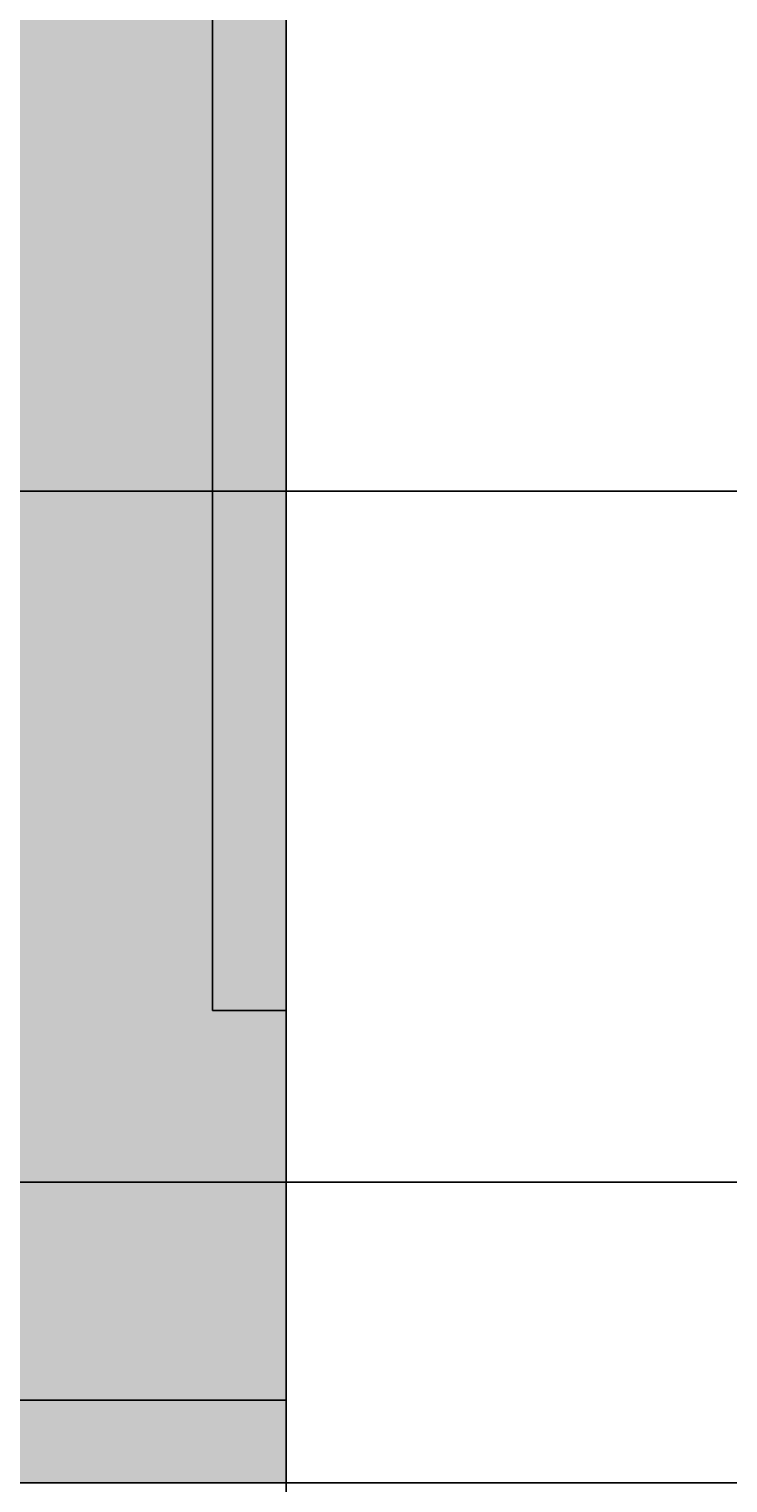
# Model space of a CAD drawing. Units: feet. Extents: x 2193 to 3502, y 890 to 1601.
# Tile 7 of 17: x 2710 to 2848, y 1073 to 1360. Entities that reach past the tile are written whole.
import ezdxf

# ---------------------------------------------------------------- set-up
doc = ezdxf.new("R2010")
doc.units = ezdxf.units.FT
for name, color, linetype, lineweight in [('A-ANNO-DIMS', 2, 'Continuous', 18), ('A-ELEV', 7, 'Continuous', 25), ('A-ELEV-PATT', 8, 'Continuous', 13)]:
    doc.layers.add(name, color=color, linetype=linetype, lineweight=lineweight)
doc.styles.get("Standard").update_dxf_attribs({"font": 'arial.ttf'})
doc.dimstyles.get("Standard").update_dxf_attribs({"dimtxt": 0.18, "dimasz": 0.18, "dimexe": 0.18, "dimexo": 0.0625, "dimgap": 0.09, "dimtad": 0, "dimtih": 1, "dimtoh": 1, "dimdec": 0, "dimzin": 0, "dimdsep": 46, "dimlunit": 3, "dimtxsty": 'Standard', "dimcen": 0.09, "dimadec": 0, "dimazin": 0, "dimtfac": 1, "dimtdec": 0, "dimtofl": 0, "dimtmove": 0, "dimatfit": 3, "dimfxl": 1, "dimtolj": 1, "dimtzin": 0, "dimarcsym": 0})

# ---------------------------------------------------------------- blocks, each defined once
blk = doc.blocks.new('*D19')
at = {"layer": 'A-ANNO-DIMS', "color": 0, "lineweight": -2, "transparency": 16777216}
for p, q in [((2934.31, 1073.03), (2193.56, 1073.03)), ((2193.74, 1072.85), (2193.74, 1012.11)), ((2193.74, 951), (2193.74, 1011.75)), ((2934.31, 950.82), (2193.56, 950.82))]:
    blk.add_line(p, q, dxfattribs=at)
at = {"layer": 'A-ANNO-DIMS', "color": 0, "transparency": 16777216}
for points in [[(2193.71, 1072.85), (2193.77, 1072.85), (2193.74, 1073.03)], [(2193.71, 951), (2193.77, 951), (2193.74, 950.82)]]:
    blk.add_solid(points, dxfattribs=at)
at = {"layer": 'Defpoints', "color": 0, "transparency": 16777216}
for p in [(2193.74, 1073.03), (2934.37, 1073.03), (2934.37, 950.82)]:
    blk.add_point(p, dxfattribs=at)
at = {"layer": 'A-ANNO-DIMS', "color": 0, "transparency": 16777216, "insert": (2193.74, 1011.93), "char_height": 0.18, "attachment_point": 5}
blk.add_mtext('\\A1;122.2', dxfattribs=at)
blk = doc.blocks.new('*D20')
at = {"layer": 'A-ANNO-DIMS', "color": 0, "lineweight": -2, "transparency": 16777216}
for p, q in [((2933.15, 1408.48), (2193.56, 1408.48)), ((2193.74, 1408.3), (2193.74, 1240.94)), ((2193.74, 1073.21), (2193.74, 1240.57)), ((2934.31, 1073.03), (2193.56, 1073.03))]:
    blk.add_line(p, q, dxfattribs=at)
at = {"layer": 'A-ANNO-DIMS', "color": 0, "transparency": 16777216}
for points in [[(2193.71, 1408.3), (2193.77, 1408.3), (2193.74, 1408.48)], [(2193.71, 1073.21), (2193.77, 1073.21), (2193.74, 1073.03)]]:
    blk.add_solid(points, dxfattribs=at)
at = {"layer": 'Defpoints', "color": 0, "transparency": 16777216}
for p in [(2193.74, 1408.48), (2933.21, 1408.48), (2934.37, 1073.03)]:
    blk.add_point(p, dxfattribs=at)
at = {"layer": 'A-ANNO-DIMS', "color": 0, "transparency": 16777216, "insert": (2193.74, 1240.76), "char_height": 0.18, "attachment_point": 5}
blk.add_mtext('\\A1;335.45', dxfattribs=at)
blk = doc.blocks.new('*D26')
at = {"layer": 'A-ANNO-DIMS', "color": 0, "lineweight": -2, "transparency": 16777216}
for p, q in [((2255.16, 950.89), (2255.16, 1601.47)), ((2255.34, 1601.29), (2507.42, 1601.29)), ((2760.29, 1601.29), (2508.21, 1601.29)), ((2760.47, 1541.11), (2760.47, 1601.47))]:
    blk.add_line(p, q, dxfattribs=at)
at = {"layer": 'A-ANNO-DIMS', "color": 0, "transparency": 16777216}
for points in [[(2255.34, 1601.32), (2255.34, 1601.26), (2255.16, 1601.29)], [(2760.29, 1601.32), (2760.29, 1601.26), (2760.47, 1601.29)]]:
    blk.add_solid(points, dxfattribs=at)
at = {"layer": 'Defpoints', "color": 0, "transparency": 16777216}
for p in [(2760.47, 1601.29), (2760.47, 1541.04), (2255.16, 950.82)]:
    blk.add_point(p, dxfattribs=at)
at = {"layer": 'A-ANNO-DIMS', "color": 0, "transparency": 16777216, "insert": (2507.82, 1601.29), "char_height": 0.18, "attachment_point": 5}
blk.add_mtext('\\A1;505.3', dxfattribs=at)
blk = doc.blocks.new('*D31')
at = {"layer": 'A-ANNO-DIMS', "color": 0, "lineweight": -2, "transparency": 16777216}
for p, q in [((2760.54, 1541.04), (3501.85, 1541.04)), ((3501.67, 1540.86), (3501.67, 1246.12)), ((3501.67, 951), (3501.67, 1245.75)), ((2762.27, 950.82), (3501.85, 950.82))]:
    blk.add_line(p, q, dxfattribs=at)
at = {"layer": 'A-ANNO-DIMS', "color": 0, "transparency": 16777216}
for points in [[(3501.64, 1540.86), (3501.7, 1540.86), (3501.67, 1541.04)], [(3501.64, 951), (3501.7, 951), (3501.67, 950.82)]]:
    blk.add_solid(points, dxfattribs=at)
at = {"layer": 'Defpoints', "color": 0, "transparency": 16777216}
for p in [(2760.47, 1541.04), (3501.67, 1541.04), (2762.2, 950.82)]:
    blk.add_point(p, dxfattribs=at)
at = {"layer": 'A-ANNO-DIMS', "color": 0, "transparency": 16777216, "insert": (3501.67, 1245.93), "char_height": 0.18, "attachment_point": 5}
blk.add_mtext('\\A1;590.2', dxfattribs=at)
blk = doc.blocks.new('*D35')
at = {"layer": 'A-ANNO-DIMS', "color": 0, "lineweight": -2, "transparency": 16777216}
for p, q in [((2980.65, 1132.39), (2193.56, 1132.39)), ((2193.74, 1132.21), (2193.74, 1102.89)), ((2193.74, 1073.21), (2193.74, 1102.53)), ((2934.31, 1073.03), (2193.56, 1073.03))]:
    blk.add_line(p, q, dxfattribs=at)
at = {"layer": 'A-ANNO-DIMS', "color": 0, "transparency": 16777216}
for points in [[(2193.71, 1132.21), (2193.77, 1132.21), (2193.74, 1132.39)], [(2193.71, 1073.21), (2193.77, 1073.21), (2193.74, 1073.03)]]:
    blk.add_solid(points, dxfattribs=at)
at = {"layer": 'Defpoints', "color": 0, "transparency": 16777216}
for p in [(2193.74, 1132.39), (2980.72, 1132.39), (2934.37, 1073.03)]:
    blk.add_point(p, dxfattribs=at)
at = {"layer": 'A-ANNO-DIMS', "color": 0, "transparency": 16777216, "insert": (2193.74, 1102.71), "char_height": 0.18, "attachment_point": 5}
blk.add_mtext('\\A1;59.36', dxfattribs=at)
blk = doc.blocks.new('*D36')
at = {"layer": 'A-ANNO-DIMS', "color": 0, "lineweight": -2, "transparency": 16777216}
for p, q in [((2974.05, 1268.66), (2193.56, 1268.66)), ((2193.74, 1268.48), (2193.74, 1200.71)), ((2193.74, 1132.57), (2193.74, 1200.34)), ((2980.65, 1132.39), (2193.56, 1132.39))]:
    blk.add_line(p, q, dxfattribs=at)
at = {"layer": 'A-ANNO-DIMS', "color": 0, "transparency": 16777216}
for points in [[(2193.71, 1268.48), (2193.77, 1268.48), (2193.74, 1268.66)], [(2193.71, 1132.57), (2193.77, 1132.57), (2193.74, 1132.39)]]:
    blk.add_solid(points, dxfattribs=at)
at = {"layer": 'Defpoints', "color": 0, "transparency": 16777216}
for p in [(2193.74, 1268.66), (2974.12, 1268.66), (2980.72, 1132.39)]:
    blk.add_point(p, dxfattribs=at)
at = {"layer": 'A-ANNO-DIMS', "color": 0, "transparency": 16777216, "insert": (2193.74, 1200.53), "char_height": 0.18, "attachment_point": 5}
blk.add_mtext('\\A1;136.27', dxfattribs=at)
blk = doc.blocks.new('*D37')
at = {"layer": 'A-ANNO-DIMS', "color": 0, "lineweight": -2, "transparency": 16777216}
for p, q in [((2974.05, 1367.57), (2193.56, 1367.57)), ((2193.74, 1367.39), (2193.74, 1318.3)), ((2193.74, 1268.84), (2193.74, 1317.93)), ((2974.05, 1268.66), (2193.56, 1268.66))]:
    blk.add_line(p, q, dxfattribs=at)
at = {"layer": 'A-ANNO-DIMS', "color": 0, "transparency": 16777216}
for points in [[(2193.71, 1367.39), (2193.77, 1367.39), (2193.74, 1367.57)], [(2193.71, 1268.84), (2193.77, 1268.84), (2193.74, 1268.66)]]:
    blk.add_solid(points, dxfattribs=at)
at = {"layer": 'Defpoints', "color": 0, "transparency": 16777216}
for p in [(2193.74, 1367.57), (2974.12, 1367.57), (2974.12, 1268.66)]:
    blk.add_point(p, dxfattribs=at)
at = {"layer": 'A-ANNO-DIMS', "color": 0, "transparency": 16777216, "insert": (2193.74, 1318.12), "char_height": 0.18, "attachment_point": 5}
blk.add_mtext('\\A1;98.91', dxfattribs=at)

msp = doc.modelspace()

# ---------------------------------------------------------------- hatches: boundary and pattern name
at = {"layer": 'A-ELEV-PATT'}
h = msp.add_hatch(color=256, dxfattribs=at)
h.dxf.hatch_style = 1
h.paths.add_polyline_path([(2760.4733, 1541.0441), (2699.6322, 1541.0441), (2699.6322, 1512.3957), (2760.4733, 1512.3957)])
h.paths.add_polyline_path([(2760.4733, 1502.0763), (2699.6322, 1502.0763), (2699.6322, 1382.0763), (2760.4733, 1382.0763)])
h.paths.add_polyline_path([(2745.971, 1367.5739), (2699.6322, 1367.5739), (2699.6322, 1089.3627), (2760.4733, 1089.3627), (2760.4733, 1166.2327), (2745.971, 1166.2327)])
h.paths.add_polyline_path([(2754.7661, 1011.1246), (2690.9216, 1011.1246), (2690.9216, 993.3923), (2754.7661, 993.3923)])
h.paths.add_polyline_path([(2689.6008, 1011.1246), (2625.7563, 1011.1246), (2625.7563, 993.3923), (2689.6008, 993.3923)])
h.paths.add_polyline_path([(2599.6883, 1249.8256), (2598.591, 1249.8256), (2598.591, 1233.561), (2599.6883, 1233.561)])
h.paths.add_polyline_path([(2602.5204, 1247.0422), (2601.423, 1247.0422), (2601.423, 1233.561), (2602.5204, 1233.561)])
h.paths.add_polyline_path([(2606.5316, 1250.4403), (2605.4342, 1250.4403), (2605.4342, 1233.561), (2606.5316, 1233.561)])
h.paths.add_polyline_path([(2609.5836, 1248.4363), (2608.4862, 1248.4363), (2608.4862, 1233.561), (2609.5836, 1233.561)])
h.paths.add_polyline_path([(2613.8564, 1243.2956), (2612.759, 1243.2956), (2612.759, 1233.561), (2613.8564, 1233.561)])
h.paths.add_polyline_path([(2616.5596, 1249.6561), (2615.4622, 1249.6561), (2615.4622, 1233.561), (2616.5596, 1233.561)])
h.paths.add_polyline_path([(2599.6883, 1233.561), (2598.591, 1233.561), (2598.591, 1224.865), (2599.6883, 1224.865)])
h.paths.add_polyline_path([(2602.5204, 1233.561), (2601.423, 1233.561), (2601.423, 1224.865), (2602.5204, 1224.865)])
h.paths.add_polyline_path([(2606.5316, 1233.561), (2605.4342, 1233.561), (2605.4342, 1224.865), (2606.5316, 1224.865)])
h.paths.add_polyline_path([(2609.5836, 1233.561), (2608.4862, 1233.561), (2608.4862, 1224.865), (2609.5836, 1224.865)])
h.paths.add_polyline_path([(2613.8564, 1233.561), (2612.759, 1233.561), (2612.759, 1224.865), (2613.8564, 1224.865)])
h.paths.add_polyline_path([(2616.5596, 1233.561), (2615.4622, 1233.561), (2615.4622, 1224.865), (2616.5596, 1224.865)])
h.paths.add_polyline_path([(2599.6883, 1224.865), (2598.591, 1224.865), (2598.591, 1115.2331), (2599.6883, 1115.2331)])
h.paths.add_polyline_path([(2602.5204, 1224.865), (2601.423, 1224.865), (2601.423, 1112.4498), (2602.5204, 1112.4498)])
h.paths.add_polyline_path([(2606.5316, 1224.865), (2605.4342, 1224.865), (2605.4342, 1115.8479), (2606.5316, 1115.8479)])
h.paths.add_polyline_path([(2609.5836, 1224.865), (2608.4862, 1224.865), (2608.4862, 1113.8439), (2609.5836, 1113.8439)])
h.paths.add_polyline_path([(2616.5596, 1224.865), (2615.4622, 1224.865), (2615.4622, 1115.0637), (2616.5596, 1115.0637)])
h.paths.add_polyline_path([(2613.8564, 1224.865), (2612.759, 1224.865), (2612.759, 1108.7032), (2613.8564, 1108.7032)])
h = msp.add_hatch(color=256, dxfattribs=at)
h.dxf.hatch_style = 1
h.paths.add_polyline_path([(2760.4733, 1512.3957), (2586.1736, 1512.3957), (2586.1736, 1502.0763), (2602.8648, 1502.0763), (2699.5726, 1502.0763), (2699.6322, 1502.0763), (2760.4733, 1502.0763)])
h.paths.add_polyline_path([(2760.4733, 1382.0763), (2275.0482, 1382.0763), (2275.0482, 1367.5739), (2745.971, 1367.5739), (2745.971, 1166.2327), (2760.4733, 1166.2327)])
h.paths.add_polyline_path([(2468.2854, 1266.7092), (2294.8992, 1266.7092), (2294.8992, 1079.031), (2468.2854, 1079.031)])
h.paths.add_polyline_path([(2301.4984, 1260.11), (2461.6863, 1260.11), (2461.6863, 1085.6301), (2301.4984, 1085.6301)], flags=16)
h.paths.add_polyline_path([(2452.7821, 1241.1967), (2452.7821, 1217.2819), (2454.6216, 1217.2819), (2454.6216, 1133.1367), (2461.6863, 1133.1367), (2461.6863, 1132.3937), (2381.7172, 1132.3937), (2381.7172, 1085.6301), (2381.4675, 1085.6301), (2381.4675, 1132.3937), (2301.4984, 1132.3937), (2301.4984, 1133.1367), (2301.4984, 1217.2819), (2390.8933, 1217.2819), (2390.8933, 1241.1967)], flags=0)
h.paths.add_polyline_path([(2372.4936, 1214.8367), (2372.4936, 1133.1367), (2371.1246, 1133.1367), (2371.1246, 1214.8367), (2337.2323, 1214.8367), (2337.2323, 1133.1367), (2335.8632, 1133.1367), (2335.8632, 1214.8367), (2337.2323, 1214.8367)], flags=0)
h = msp.add_hatch(color=256, dxfattribs=at)
h.dxf.hatch_style = 1
h.paths.add_polyline_path([(2294.8992, 1367.5739), (2275.0482, 1367.5739), (2275.0482, 1382.0763), (2536.5416, 1382.0763), (2536.5416, 1406.15), (2256.3232, 1406.15), (2256.3232, 1089.3627), (2255.1574, 1089.3627), (2255.1574, 1073.031), (2294.8992, 1073.031)])
h.paths.add_polyline_path([(2517.7591, 1241.1967), (2468.2854, 1241.1967), (2468.2854, 1224.865), (2598.591, 1224.865), (2598.591, 1233.561), (2517.7591, 1233.561)])
h.paths.add_polyline_path([(2699.6322, 1241.1967), (2636.5184, 1241.1967), (2636.5184, 1233.561), (2616.5596, 1233.561), (2616.5596, 1224.865), (2699.6322, 1224.865)])
h.paths.add_polyline_path([(2615.4622, 1233.561), (2613.8564, 1233.561), (2613.8564, 1224.865), (2615.4622, 1224.865)])
h.paths.add_polyline_path([(2612.759, 1233.561), (2609.5836, 1233.561), (2609.5836, 1224.865), (2612.759, 1224.865)])
h.paths.add_polyline_path([(2608.4862, 1233.561), (2606.5316, 1233.561), (2606.5316, 1224.865), (2608.4862, 1224.865)])
h.paths.add_polyline_path([(2605.4342, 1233.561), (2602.5204, 1233.561), (2602.5204, 1224.865), (2605.4342, 1224.865)])
h.paths.add_polyline_path([(2601.423, 1233.561), (2599.6883, 1233.561), (2599.6883, 1224.865), (2601.423, 1224.865)])
h.paths.add_polyline_path([(2517.7591, 1089.3627), (2468.2854, 1089.3627), (2468.2854, 1079.031), (2294.8992, 1079.031), (2294.8992, 1073.031), (2390.8933, 1073.031), (2452.7821, 1073.031), (2760.4733, 1073.031), (2760.4733, 1089.3627), (2699.6322, 1089.3627), (2636.5184, 1089.3627), (2636.5184, 1081.7269), (2517.7591, 1081.7269)])

# ---------------------------------------------------------------- linework, layer by layer
at = {"layer": 'A-ELEV'}
for p, q in [((2760.4733, 956.8829), (2760.4733, 1494.0584)), ((2745.971, 1166.2327), (2760.4733, 1166.2327)), ((2636.5184, 1089.3627), (2760.4733, 1089.3627)), ((2636.5184, 1089.3627), (2760.4733, 1089.3627))]:
    msp.add_line(p, q, dxfattribs=at)
for points in [[(2760.4733, 1494.0584), (2760.4733, 956.8829), (2762.2048, 950.8228), (2626.1971, 950.8228), (2255.1574, 950.8228), (2255.1574, 953.031), (2255.1574, 1073.031), (2260.8647, 1073.031), (2260.8647, 956.5285)], [(2760.4733, 1415.3157), (2760.4733, 1089.3627), (2699.6322, 1089.3627), (2699.6322, 1367.5739)], [(2760.4733, 1415.3157), (2760.4733, 1089.3627), (2699.6322, 1089.3627), (2699.6322, 1367.5739)], [(2760.4733, 1166.2327), (2745.971, 1166.2327), (2745.971, 1367.5739), (2275.0482, 1367.5739), (2275.0482, 1382.0763), (2760.4733, 1382.0763), (2760.4733, 1367.5739)], [(2745.971, 1166.2327), (2745.971, 1367.5739)]]:
    msp.add_lwpolyline(points, dxfattribs=at)

# ---------------------------------------------------------------- dimensions: what is measured, and where the dimension line sits
at = {"layer": 'A-ANNO-DIMS'}
dim = msp.add_linear_dim(base=(2760.4733, 1601.2941), p1=(2255.1574, 950.8228), p2=(2760.4733, 1541.0441), dimstyle='Standard', override={"dimdec": 1, "dimlfac": 1, "dimrnd": 0, "dimzin": 0, "dimdsep": 46, "dimlunit": 2}, dxfattribs=at)
dim.commit()
dim.dimension.update_dxf_attribs({"geometry": '*D26', "text_midpoint": (2507.8154, 1601.2941)})
for base, p1, p2, override, picture, middle in [((3501.6716, 1541.0441), (2762.2048, 950.8228), (2760.4733, 1541.0441), {"dimdec": 1, "dimlfac": 1, "dimrnd": 0, "dimzin": 0, "dimdsep": 46, "dimlunit": 2}, '*D31', (3501.6716, 1245.9334)), ((2193.7417, 1408.4814), (2934.3742, 1073.031), (2933.2085, 1408.4814), {"dimdec": 2, "dimlfac": 1, "dimrnd": 0, "dimzin": 0, "dimdsep": 46, "dimlunit": 2}, '*D20', (2193.7417, 1240.7562)), ((2193.7417, 1367.5739), (2974.116, 1268.6599), (2974.116, 1367.5739), {"dimdec": 2, "dimlfac": 1, "dimrnd": 0, "dimzin": 0, "dimdsep": 46, "dimlunit": 2}, '*D37', (2193.7417, 1318.1169)), ((2193.7417, 1268.6599), (2980.7151, 1132.3937), (2974.116, 1268.6599), {"dimdec": 2, "dimlfac": 1, "dimrnd": 0, "dimzin": 0, "dimdsep": 46, "dimlunit": 2}, '*D36', (2193.7417, 1200.5268)), ((2193.7417, 1132.3937), (2934.3742, 1073.031), (2980.7151, 1132.3937), {"dimdec": 2, "dimlfac": 1, "dimrnd": 0, "dimzin": 0, "dimdsep": 46, "dimlunit": 2}, '*D35', (2193.7417, 1102.7124)), ((2193.7417, 1073.031), (2934.3742, 950.8228), (2934.3742, 1073.031), {"dimdec": 1, "dimlfac": 1, "dimrnd": 0, "dimzin": 0, "dimdsep": 46, "dimlunit": 2}, '*D19', (2193.7417, 1011.9269))]:
    dim = msp.add_linear_dim(base=base, p1=p1, p2=p2, angle=90, dimstyle='Standard', override=override, dxfattribs=at)
    dim.commit()
    dim.dimension.update_dxf_attribs({"geometry": picture, "text_midpoint": middle})

doc.saveas('drawing.dxf')
